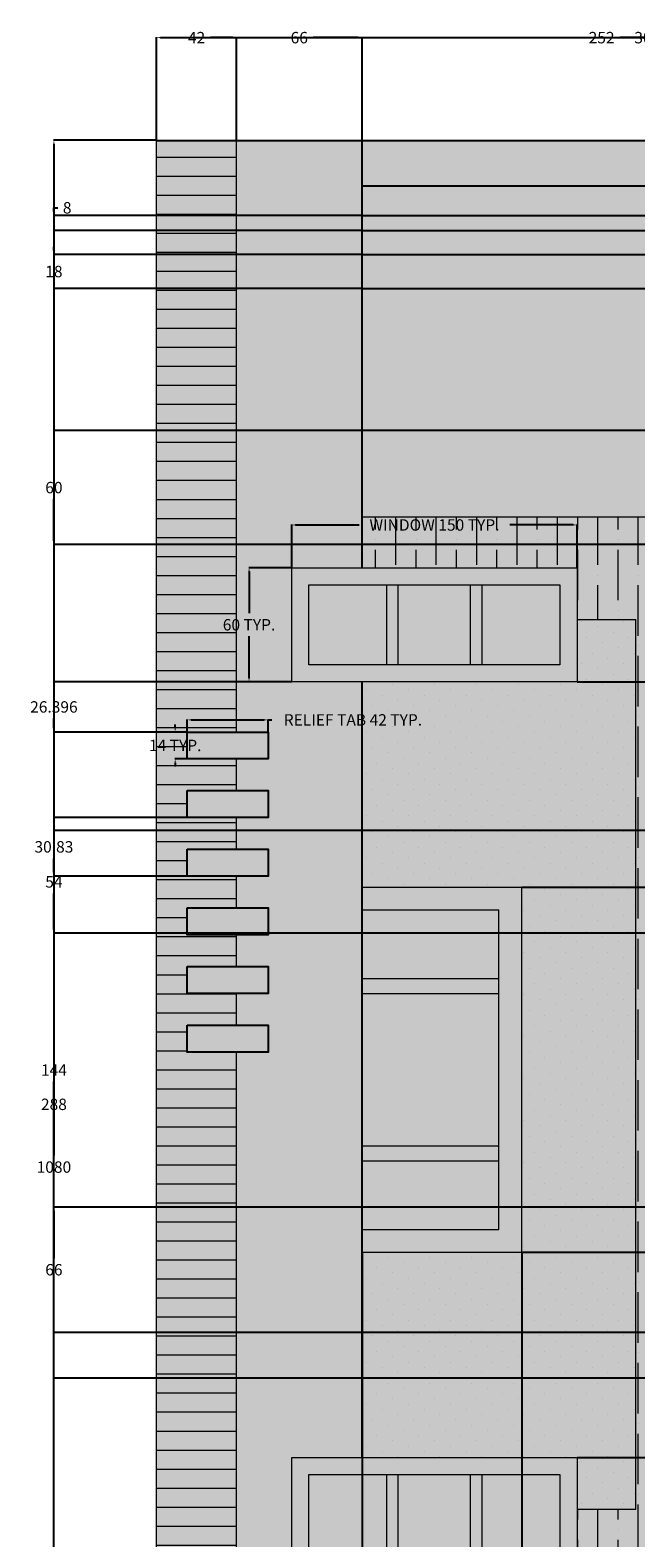
# Model space of a CAD drawing. Units: inches. Extents: x 180 to 1069, y 71 to 1267.
# Tile 6 of 8: x 180 to 498, y 474 to 1267. Entities that reach past the tile are written whole.
import ezdxf

# ---------------------------------------------------------------- set-up
doc = ezdxf.new("R2010")
doc.units = ezdxf.units.IN
doc.header["$MEASUREMENT"] = 0
for name, color, linetype, lineweight in [('A-ANNO-DIMS', 2, 'Continuous', 18), ('A-ELEV-FRAM', 7, 'Continuous', 25), ('A-GLAZ', 7, 'Continuous', 18), ('A-WALL-CLAD', 7, 'Continuous', 18), ('A-WALL-CLAD-JNTS-PATT', 18, 'Continuous', 13), ('A-WALL-CLAD-PATT', 26, 'Continuous', 13), ('A-WALL-SCRN-JNTS-PATT', 8, 'Continuous', 13)]:
    doc.layers.add(name, color=color, linetype=linetype, lineweight=lineweight)
for name, color, linetype, lineweight, true_color in [('A-ELEV-BAND-PATT', 30, 'Continuous', 13, 0xf26722), ('A-ELEV-FRAM-PATT', 53, 'Continuous', 13, 0xefd648), ('A-ELEV-REVL-PATT', 9, 'Continuous', 13, 0xc7c8ca), ('A-ELEV-TRIM-PATT', 7, 'Continuous', 13, 0xffffff), ('A-WALL-PANL-PATT', 252, 'Continuous', 13, 0x939598), ('A-WALL-SCRN-PATT', 251, 'Continuous', 13, 0x636466), ('A-WALL-STUC-PATT', 9, 'Continuous', 13, 0xc7c8ca)]:
    doc.layers.add(name, color=color, linetype=linetype, lineweight=lineweight, true_color=true_color)
doc.styles.get("Standard").update_dxf_attribs({"font": 'arial.ttf'})
doc.dimstyles.get("Standard").update_dxf_attribs({"dimtxt": 6, "dimasz": 2, "dimexe": 0.18, "dimexo": 0.0625, "dimgap": 3, "dimtad": 0, "dimtih": 1, "dimtoh": 1, "dimdec": 0, "dimzin": 0, "dimdsep": 46, "dimlunit": 3, "dimtxsty": 'Standard', "dimcen": 0.09, "dimadec": 0, "dimazin": 0, "dimtfac": 1, "dimtdec": 0, "dimtofl": 0, "dimtmove": 0, "dimatfit": 3, "dimfxl": 1, "dimtolj": 1, "dimtzin": 0, "dimarcsym": 0})

# ---------------------------------------------------------------- blocks, each defined once
blk = doc.blocks.new('WIN-THREE-LIGHT')
for p, q in [((50, 9), (50, 51)), ((56, 9), (56, 51)), ((94, 9), (94, 51)), ((100, 9), (100, 51))]:
    blk.add_line(p, q)
for points in [[(0, 60), (150, 60), (150, 0), (0, 0)], [(9, 51), (141, 51), (141, 9), (9, 9)]]:
    blk.add_lwpolyline(points, close=True)
blk = doc.blocks.new('FACADE-RELIEF-TAB')
blk.add_lwpolyline([(0, 14.15), (42.5, 14.15), (42.5, 0), (0, 0)], close=True)
blk = doc.blocks.new('*D8')
at = {"layer": 'A-ANNO-DIMS', "color": 0, "lineweight": -2, "transparency": 16777216}
for p, q in [((262.22, 897.7), (262.22, 904.19)), ((264.22, 904.01), (302.72, 904.01)), ((304.72, 897.7), (304.72, 904.19)), ((304.72, 904.01), (306.72, 904.01))]:
    blk.add_line(p, q, dxfattribs=at)
at = {"layer": 'A-ANNO-DIMS', "color": 0, "transparency": 16777216}
for points in [[(264.22, 904.34), (264.22, 903.68), (262.22, 904.01)], [(302.72, 904.34), (302.72, 903.68), (304.72, 904.01)]]:
    blk.add_solid(points, dxfattribs=at)
at = {"layer": 'Defpoints', "color": 0, "transparency": 16777216}
for p in [(304.72, 904.01), (262.22, 897.63), (304.72, 897.63)]:
    blk.add_point(p, dxfattribs=at)
at = {"layer": 'A-ANNO-DIMS', "color": 0, "transparency": 16777216, "insert": (349.32, 904.01), "char_height": 6, "attachment_point": 5}
blk.add_mtext('\\A1;RELIEF TAB 42 TYP.', dxfattribs=at)
blk = doc.blocks.new('*D9')
at = {"layer": 'A-ANNO-DIMS', "color": 0, "lineweight": -2, "transparency": 16777216}
for p, q in [((262.16, 897.63), (255.66, 897.63)), ((255.84, 899.63), (255.84, 901.63)), ((262.16, 883.48), (255.66, 883.48)), ((255.84, 881.48), (255.84, 879.48))]:
    blk.add_line(p, q, dxfattribs=at)
at = {"layer": 'A-ANNO-DIMS', "color": 0, "transparency": 16777216}
for points in [[(255.51, 899.63), (256.18, 899.63), (255.84, 897.63)], [(255.51, 881.48), (256.18, 881.48), (255.84, 883.48)]]:
    blk.add_solid(points, dxfattribs=at)
at = {"layer": 'Defpoints', "color": 0, "transparency": 16777216}
for p in [(255.84, 897.63), (262.22, 897.63), (262.22, 883.48)]:
    blk.add_point(p, dxfattribs=at)
at = {"layer": 'A-ANNO-DIMS', "color": 0, "transparency": 16777216, "insert": (255.84, 890.56), "char_height": 6, "attachment_point": 5}
blk.add_mtext('\\A1;14 TYP.', dxfattribs=at)
blk = doc.blocks.new('*D10')
at = {"layer": 'A-ANNO-DIMS', "color": 0, "lineweight": -2, "transparency": 16777216}
for p, q in [((317.19, 984.09), (317.19, 1006.71)), ((319.19, 1006.53), (352.58, 1006.53)), ((465.19, 1006.53), (431.8, 1006.53)), ((467.19, 984.09), (467.19, 1006.71))]:
    blk.add_line(p, q, dxfattribs=at)
at = {"layer": 'A-ANNO-DIMS', "color": 0, "transparency": 16777216}
for points in [[(319.19, 1006.86), (319.19, 1006.2), (317.19, 1006.53)], [(465.19, 1006.86), (465.19, 1006.2), (467.19, 1006.53)]]:
    blk.add_solid(points, dxfattribs=at)
at = {"layer": 'Defpoints', "color": 0, "transparency": 16777216}
for p in [(467.19, 1006.53), (317.19, 984.03), (467.19, 984.03)]:
    blk.add_point(p, dxfattribs=at)
at = {"layer": 'A-ANNO-DIMS', "color": 0, "transparency": 16777216, "insert": (392.19, 1006.53), "char_height": 6, "attachment_point": 5}
blk.add_mtext('\\A1;WINDOW 150 TYP.', dxfattribs=at)
blk = doc.blocks.new('*D11')
at = {"layer": 'A-ANNO-DIMS', "color": 0, "lineweight": -2, "transparency": 16777216}
for p, q in [((317.13, 984.03), (294.51, 984.03)), ((294.69, 982.03), (294.69, 960.09)), ((294.69, 926.03), (294.69, 947.97)), ((317.13, 924.03), (294.51, 924.03))]:
    blk.add_line(p, q, dxfattribs=at)
at = {"layer": 'A-ANNO-DIMS', "color": 0, "transparency": 16777216}
for points in [[(294.36, 982.03), (295.02, 982.03), (294.69, 984.03)], [(294.36, 926.03), (295.02, 926.03), (294.69, 924.03)]]:
    blk.add_solid(points, dxfattribs=at)
at = {"layer": 'Defpoints', "color": 0, "transparency": 16777216}
for p in [(294.69, 984.03), (317.19, 984.03), (317.19, 924.03)]:
    blk.add_point(p, dxfattribs=at)
at = {"layer": 'A-ANNO-DIMS', "color": 0, "transparency": 16777216, "insert": (294.69, 954.03), "char_height": 6, "attachment_point": 5}
blk.add_mtext('\\A1;60 TYP.', dxfattribs=at)
blk = doc.blocks.new('*D16')
at = {"layer": 'A-ANNO-DIMS', "color": 0, "lineweight": -2, "transparency": 16777216}
for p, q in [((246.09, 1208.88), (246.09, 1263.01)), ((248.09, 1262.83), (614.49, 1262.83)), ((1000.09, 1262.83), (633.69, 1262.83)), ((1002.09, 1148.88), (1002.09, 1263.01))]:
    blk.add_line(p, q, dxfattribs=at)
at = {"layer": 'A-ANNO-DIMS', "color": 0, "transparency": 16777216}
for points in [[(248.09, 1263.16), (248.09, 1262.5), (246.09, 1262.83)], [(1000.09, 1263.16), (1000.09, 1262.5), (1002.09, 1262.83)]]:
    blk.add_solid(points, dxfattribs=at)
at = {"layer": 'Defpoints', "color": 0, "transparency": 16777216}
for p in [(1002.09, 1262.83), (246.09, 1208.82), (1002.09, 1148.82)]:
    blk.add_point(p, dxfattribs=at)
at = {"layer": 'A-ANNO-DIMS', "color": 0, "transparency": 16777216, "insert": (624.09, 1262.83), "char_height": 6, "attachment_point": 5}
blk.add_mtext('\\A1;756', dxfattribs=at)
blk = doc.blocks.new('*D17')
at = {"layer": 'A-ANNO-DIMS', "color": 0, "lineweight": -2, "transparency": 16777216}
for p, q in [((246.02, 1208.82), (191.89, 1208.82)), ((192.07, 1206.82), (192.07, 674.88)), ((192.07, 130.82), (192.07, 662.75)), ((246.02, 128.82), (191.89, 128.82))]:
    blk.add_line(p, q, dxfattribs=at)
at = {"layer": 'A-ANNO-DIMS', "color": 0, "transparency": 16777216}
for points in [[(191.74, 1206.82), (192.41, 1206.82), (192.07, 1208.82)], [(191.74, 130.82), (192.41, 130.82), (192.07, 128.82)]]:
    blk.add_solid(points, dxfattribs=at)
at = {"layer": 'Defpoints', "color": 0, "transparency": 16777216}
for p in [(192.07, 1208.82), (246.09, 1208.82), (246.09, 128.82)]:
    blk.add_point(p, dxfattribs=at)
at = {"layer": 'A-ANNO-DIMS', "color": 0, "transparency": 16777216, "insert": (192.07, 668.82), "char_height": 6, "attachment_point": 5}
blk.add_mtext('\\A1;1080', dxfattribs=at)
blk = doc.blocks.new('*D19')
at = {"layer": 'A-ANNO-DIMS', "color": 0, "lineweight": -2, "transparency": 16777216}
for p, q in [((246.09, 1208.88), (246.09, 1263.01)), ((248.09, 1262.83), (259.7, 1262.83)), ((286.09, 1262.83), (274.47, 1262.83)), ((288.09, 1208.88), (288.09, 1263.01))]:
    blk.add_line(p, q, dxfattribs=at)
at = {"layer": 'A-ANNO-DIMS', "color": 0, "transparency": 16777216}
for points in [[(248.09, 1263.16), (248.09, 1262.5), (246.09, 1262.83)], [(286.09, 1263.16), (286.09, 1262.5), (288.09, 1262.83)]]:
    blk.add_solid(points, dxfattribs=at)
at = {"layer": 'Defpoints', "color": 0, "transparency": 16777216}
for p in [(288.09, 1262.83), (246.09, 1208.82), (288.09, 1208.82)]:
    blk.add_point(p, dxfattribs=at)
at = {"layer": 'A-ANNO-DIMS', "color": 0, "transparency": 16777216, "insert": (267.09, 1262.83), "char_height": 6, "attachment_point": 5}
blk.add_mtext('\\A1;42', dxfattribs=at)
blk = doc.blocks.new('*D20')
at = {"layer": 'A-ANNO-DIMS', "color": 0, "lineweight": -2, "transparency": 16777216}
for p, q in [((288.09, 1208.88), (288.09, 1263.01)), ((290.09, 1262.83), (313.78, 1262.83)), ((352.09, 1262.83), (328.4, 1262.83)), ((354.09, 1184.88), (354.09, 1263.01))]:
    blk.add_line(p, q, dxfattribs=at)
at = {"layer": 'A-ANNO-DIMS', "color": 0, "transparency": 16777216}
for points in [[(290.09, 1263.16), (290.09, 1262.5), (288.09, 1262.83)], [(352.09, 1263.16), (352.09, 1262.5), (354.09, 1262.83)]]:
    blk.add_solid(points, dxfattribs=at)
at = {"layer": 'Defpoints', "color": 0, "transparency": 16777216}
for p in [(354.09, 1262.83), (288.09, 1208.82), (354.09, 1184.82)]:
    blk.add_point(p, dxfattribs=at)
at = {"layer": 'A-ANNO-DIMS', "color": 0, "transparency": 16777216, "insert": (321.09, 1262.83), "char_height": 6, "attachment_point": 5}
blk.add_mtext('\\A1;66', dxfattribs=at)
blk = doc.blocks.new('*D21')
at = {"layer": 'A-ANNO-DIMS', "color": 0, "lineweight": -2, "transparency": 16777216}
for p, q in [((354.09, 1184.88), (354.09, 1263.01)), ((356.09, 1262.83), (494.47, 1262.83)), ((652.09, 1262.83), (513.7, 1262.83)), ((654.09, 1184.88), (654.09, 1263.01))]:
    blk.add_line(p, q, dxfattribs=at)
at = {"layer": 'A-ANNO-DIMS', "color": 0, "transparency": 16777216}
for points in [[(356.09, 1263.16), (356.09, 1262.5), (354.09, 1262.83)], [(652.09, 1263.16), (652.09, 1262.5), (654.09, 1262.83)]]:
    blk.add_solid(points, dxfattribs=at)
at = {"layer": 'Defpoints', "color": 0, "transparency": 16777216}
for p in [(654.09, 1262.83), (354.09, 1184.82), (654.09, 1184.82)]:
    blk.add_point(p, dxfattribs=at)
at = {"layer": 'A-ANNO-DIMS', "color": 0, "transparency": 16777216, "insert": (504.09, 1262.83), "char_height": 6, "attachment_point": 5}
blk.add_mtext('\\A1;300', dxfattribs=at)
blk = doc.blocks.new('*D25')
at = {"layer": 'A-ANNO-DIMS', "color": 0, "lineweight": -2, "transparency": 16777216}
for p, q in [((354.02, 1169.34), (191.89, 1169.34)), ((192.07, 1171.34), (192.07, 1173.34)), ((192.07, 1173.34), (194.07, 1173.34)), ((354.02, 1161.34), (191.89, 1161.34)), ((192.07, 1159.34), (192.07, 1157.34))]:
    blk.add_line(p, q, dxfattribs=at)
at = {"layer": 'A-ANNO-DIMS', "color": 0, "transparency": 16777216}
for points in [[(191.74, 1171.34), (192.41, 1171.34), (192.07, 1169.34)], [(191.74, 1159.34), (192.41, 1159.34), (192.07, 1161.34)]]:
    blk.add_solid(points, dxfattribs=at)
at = {"layer": 'Defpoints', "color": 0, "transparency": 16777216}
for p in [(192.07, 1169.34), (354.09, 1169.34), (354.09, 1161.34)]:
    blk.add_point(p, dxfattribs=at)
at = {"layer": 'A-ANNO-DIMS', "color": 0, "transparency": 16777216, "insert": (199.05, 1173.34), "char_height": 6, "attachment_point": 5}
blk.add_mtext('\\A1;8', dxfattribs=at)
blk = doc.blocks.new('*D27')
at = {"layer": 'A-ANNO-DIMS', "color": 0, "lineweight": -2, "transparency": 16777216}
for p, q in [((192.07, 1150.82), (192.07, 1152.82)), ((354.02, 1148.82), (191.89, 1148.82)), ((354.02, 1130.82), (191.89, 1130.82)), ((192.07, 1128.82), (192.07, 1126.82))]:
    blk.add_line(p, q, dxfattribs=at)
at = {"layer": 'A-ANNO-DIMS', "color": 0, "transparency": 16777216}
for points in [[(191.74, 1150.82), (192.41, 1150.82), (192.07, 1148.82)], [(191.74, 1128.82), (192.41, 1128.82), (192.07, 1130.82)]]:
    blk.add_solid(points, dxfattribs=at)
at = {"layer": 'Defpoints', "color": 0, "transparency": 16777216}
for p in [(192.07, 1148.82), (354.09, 1148.82), (354.09, 1130.82)]:
    blk.add_point(p, dxfattribs=at)
at = {"layer": 'A-ANNO-DIMS', "color": 0, "transparency": 16777216, "insert": (192.07, 1139.82), "char_height": 6, "attachment_point": 5}
blk.add_mtext('\\A1;18', dxfattribs=at)
blk = doc.blocks.new('*D48')
at = {"layer": 'A-ANNO-DIMS', "color": 0, "lineweight": -2, "transparency": 16777216}
for p, q in [((262.16, 852.65), (191.89, 852.65)), ((192.07, 850.65), (192.07, 843.3)), ((192.07, 823.82), (192.07, 831.17)), ((262.16, 821.82), (191.89, 821.82))]:
    blk.add_line(p, q, dxfattribs=at)
at = {"layer": 'A-ANNO-DIMS', "color": 0, "transparency": 16777216}
for points in [[(191.74, 850.65), (192.41, 850.65), (192.07, 852.65)], [(191.74, 823.82), (192.41, 823.82), (192.07, 821.82)]]:
    blk.add_solid(points, dxfattribs=at)
at = {"layer": 'Defpoints', "color": 0, "transparency": 16777216}
for p in [(262.22, 852.65), (192.07, 821.82), (262.22, 821.82)]:
    blk.add_point(p, dxfattribs=at)
at = {"layer": 'A-ANNO-DIMS', "color": 0, "transparency": 16777216, "insert": (192.07, 837.23), "char_height": 6, "attachment_point": 5}
blk.add_mtext('\\A1;30.83', dxfattribs=at)
blk = doc.blocks.new('*D49')
at = {"layer": 'A-ANNO-DIMS', "color": 0, "lineweight": -2, "transparency": 16777216}
for p, q in [((317.13, 924.03), (191.89, 924.03)), ((192.07, 922.03), (192.07, 916.9)), ((192.07, 899.63), (192.07, 904.77)), ((262.16, 897.63), (191.89, 897.63))]:
    blk.add_line(p, q, dxfattribs=at)
at = {"layer": 'A-ANNO-DIMS', "color": 0, "transparency": 16777216}
for points in [[(191.74, 922.03), (192.41, 922.03), (192.07, 924.03)], [(191.74, 899.63), (192.41, 899.63), (192.07, 897.63)]]:
    blk.add_solid(points, dxfattribs=at)
at = {"layer": 'Defpoints', "color": 0, "transparency": 16777216}
for p in [(192.07, 924.03), (317.19, 924.03), (262.22, 897.63)]:
    blk.add_point(p, dxfattribs=at)
at = {"layer": 'A-ANNO-DIMS', "color": 0, "transparency": 16777216, "insert": (192.07, 910.83), "char_height": 6, "attachment_point": 5}
blk.add_mtext('\\A1;26.396', dxfattribs=at)
blk = doc.blocks.new('*D51')
at = {"layer": 'A-ANNO-DIMS', "color": 0, "lineweight": -2, "transparency": 16777216}
for p, q in [((354.09, 624.01), (354.09, 74.62)), ((317.19, 456.06), (317.19, 74.62)), ((319.19, 74.8), (324.84, 74.8)), ((352.09, 74.8), (346.44, 74.8))]:
    blk.add_line(p, q, dxfattribs=at)
at = {"layer": 'A-ANNO-DIMS', "color": 0, "transparency": 16777216}
for points in [[(319.19, 75.14), (319.19, 74.47), (317.19, 74.8)], [(352.09, 75.14), (352.09, 74.47), (354.09, 74.8)]]:
    blk.add_solid(points, dxfattribs=at)
at = {"layer": 'Defpoints', "color": 0, "transparency": 16777216}
for p in [(354.09, 624.07), (317.19, 456.12), (354.09, 74.8)]:
    blk.add_point(p, dxfattribs=at)
at = {"layer": 'A-ANNO-DIMS', "color": 0, "transparency": 16777216, "insert": (335.64, 74.8), "char_height": 6, "attachment_point": 5}
blk.add_mtext('\\A1;36.9', dxfattribs=at)
blk = doc.blocks.new('*D52')
at = {"layer": 'A-ANNO-DIMS', "color": 0, "lineweight": -2, "transparency": 16777216}
for p, q in [((354.09, 624.01), (354.09, 74.62)), ((438.09, 624.01), (438.09, 74.62)), ((356.09, 74.8), (388.8, 74.8)), ((436.09, 74.8), (403.38, 74.8))]:
    blk.add_line(p, q, dxfattribs=at)
at = {"layer": 'A-ANNO-DIMS', "color": 0, "transparency": 16777216}
for points in [[(356.09, 75.14), (356.09, 74.47), (354.09, 74.8)], [(436.09, 75.14), (436.09, 74.47), (438.09, 74.8)]]:
    blk.add_solid(points, dxfattribs=at)
at = {"layer": 'Defpoints', "color": 0, "transparency": 16777216}
for p in [(354.09, 624.07), (438.09, 624.07), (438.09, 74.8)]:
    blk.add_point(p, dxfattribs=at)
at = {"layer": 'A-ANNO-DIMS', "color": 0, "transparency": 16777216, "insert": (396.09, 74.8), "char_height": 6, "attachment_point": 5}
blk.add_mtext('\\A1;84', dxfattribs=at)
blk = doc.blocks.new('*D53')
at = {"layer": 'A-ANNO-DIMS', "color": 0, "lineweight": -2, "transparency": 16777216}
for p, q in [((438.15, 624.07), (1056.28, 624.07)), ((1056.1, 622.07), (1056.1, 576.16)), ((1056.1, 518.12), (1056.1, 564.03)), ((467.25, 516.12), (1056.28, 516.12))]:
    blk.add_line(p, q, dxfattribs=at)
at = {"layer": 'A-ANNO-DIMS', "color": 0, "transparency": 16777216}
for points in [[(1055.77, 622.07), (1056.43, 622.07), (1056.1, 624.07)], [(1055.77, 518.12), (1056.43, 518.12), (1056.1, 516.12)]]:
    blk.add_solid(points, dxfattribs=at)
at = {"layer": 'Defpoints', "color": 0, "transparency": 16777216}
for p in [(438.09, 624.07), (1056.1, 624.07), (467.19, 516.12)]:
    blk.add_point(p, dxfattribs=at)
at = {"layer": 'A-ANNO-DIMS', "color": 0, "transparency": 16777216, "insert": (1056.1, 570.1), "char_height": 6, "attachment_point": 5}
blk.add_mtext('\\A1;107.96', dxfattribs=at)
blk = doc.blocks.new('*D54')
at = {"layer": 'A-ANNO-DIMS', "color": 0, "lineweight": -2, "transparency": 16777216}
for p, q in [((438.15, 816.07), (1056.28, 816.07)), ((1056.1, 814.07), (1056.1, 726.14)), ((1056.1, 626.07), (1056.1, 714.01)), ((438.15, 624.07), (1056.28, 624.07))]:
    blk.add_line(p, q, dxfattribs=at)
at = {"layer": 'A-ANNO-DIMS', "color": 0, "transparency": 16777216}
for points in [[(1055.77, 814.07), (1056.43, 814.07), (1056.1, 816.07)], [(1055.77, 626.07), (1056.43, 626.07), (1056.1, 624.07)]]:
    blk.add_solid(points, dxfattribs=at)
at = {"layer": 'Defpoints', "color": 0, "transparency": 16777216}
for p in [(438.09, 816.07), (1056.1, 816.07), (438.09, 624.07)]:
    blk.add_point(p, dxfattribs=at)
at = {"layer": 'A-ANNO-DIMS', "color": 0, "transparency": 16777216, "insert": (1056.1, 720.07), "char_height": 6, "attachment_point": 5}
blk.add_mtext('\\A1;192', dxfattribs=at)
blk = doc.blocks.new('*D55')
at = {"layer": 'A-ANNO-DIMS', "color": 0, "lineweight": -2, "transparency": 16777216}
for p, q in [((467.25, 924.03), (1056.28, 924.03)), ((1056.1, 922.03), (1056.1, 876.12)), ((1056.1, 818.07), (1056.1, 863.99)), ((438.15, 816.07), (1056.28, 816.07))]:
    blk.add_line(p, q, dxfattribs=at)
at = {"layer": 'A-ANNO-DIMS', "color": 0, "transparency": 16777216}
for points in [[(1055.77, 922.03), (1056.43, 922.03), (1056.1, 924.03)], [(1055.77, 818.07), (1056.43, 818.07), (1056.1, 816.07)]]:
    blk.add_solid(points, dxfattribs=at)
at = {"layer": 'Defpoints', "color": 0, "transparency": 16777216}
for p in [(467.19, 924.03), (1056.1, 924.03), (438.09, 816.07)]:
    blk.add_point(p, dxfattribs=at)
at = {"layer": 'A-ANNO-DIMS', "color": 0, "transparency": 16777216, "insert": (1056.1, 870.05), "char_height": 6, "attachment_point": 5}
blk.add_mtext('\\A1;107.96', dxfattribs=at)
blk = doc.blocks.new('*D57')
at = {"layer": 'A-ANNO-DIMS', "color": 0, "lineweight": -2, "transparency": 16777216}
for p, q in [((354.09, 1010.88), (354.09, 1263.01)), ((356.09, 1262.83), (470.44, 1262.83)), ((604.09, 1262.83), (489.74, 1262.83)), ((606.09, 1010.88), (606.09, 1263.01))]:
    blk.add_line(p, q, dxfattribs=at)
at = {"layer": 'A-ANNO-DIMS', "color": 0, "transparency": 16777216}
for points in [[(356.09, 1263.16), (356.09, 1262.5), (354.09, 1262.83)], [(604.09, 1263.16), (604.09, 1262.5), (606.09, 1262.83)]]:
    blk.add_solid(points, dxfattribs=at)
at = {"layer": 'Defpoints', "color": 0, "transparency": 16777216}
for p in [(606.09, 1262.83), (354.09, 1010.82), (606.09, 1010.82)]:
    blk.add_point(p, dxfattribs=at)
at = {"layer": 'A-ANNO-DIMS', "color": 0, "transparency": 16777216, "insert": (480.09, 1262.83), "char_height": 6, "attachment_point": 5}
blk.add_mtext('\\A1;252', dxfattribs=at)
blk = doc.blocks.new('*D62')
at = {"layer": 'A-ANNO-DIMS', "color": 0, "lineweight": -2, "transparency": 16777216}
for p, q in [((882.02, 1056.2), (191.89, 1056.2)), ((192.07, 1054.2), (192.07, 1032.26)), ((192.07, 998.2), (192.07, 1020.14)), ((882.02, 996.2), (191.89, 996.2))]:
    blk.add_line(p, q, dxfattribs=at)
at = {"layer": 'A-ANNO-DIMS', "color": 0, "transparency": 16777216}
for points in [[(191.74, 1054.2), (192.41, 1054.2), (192.07, 1056.2)], [(191.74, 998.2), (192.41, 998.2), (192.07, 996.2)]]:
    blk.add_solid(points, dxfattribs=at)
at = {"layer": 'Defpoints', "color": 0, "transparency": 16777216}
for p in [(192.07, 1056.2), (882.09, 1056.2), (882.09, 996.2)]:
    blk.add_point(p, dxfattribs=at)
at = {"layer": 'A-ANNO-DIMS', "color": 0, "transparency": 16777216, "insert": (192.07, 1026.2), "char_height": 6, "attachment_point": 5}
blk.add_mtext('\\A1;60', dxfattribs=at)
blk = doc.blocks.new('*D64')
at = {"layer": 'A-ANNO-DIMS', "color": 0, "lineweight": -2, "transparency": 16777216}
for p, q in [((612.46, 845.82), (191.89, 845.82)), ((192.07, 843.82), (192.07, 707.88)), ((192.07, 559.82), (192.07, 695.75)), ((612.46, 557.82), (191.89, 557.82))]:
    blk.add_line(p, q, dxfattribs=at)
at = {"layer": 'A-ANNO-DIMS', "color": 0, "transparency": 16777216}
for points in [[(191.74, 843.82), (192.41, 843.82), (192.07, 845.82)], [(191.74, 559.82), (192.41, 559.82), (192.07, 557.82)]]:
    blk.add_solid(points, dxfattribs=at)
at = {"layer": 'Defpoints', "color": 0, "transparency": 16777216}
for p in [(192.07, 845.82), (612.53, 845.82), (612.53, 557.82)]:
    blk.add_point(p, dxfattribs=at)
at = {"layer": 'A-ANNO-DIMS', "color": 0, "transparency": 16777216, "insert": (192.07, 701.82), "char_height": 6, "attachment_point": 5}
blk.add_mtext('\\A1;288', dxfattribs=at)
blk = doc.blocks.new('*D71')
at = {"layer": 'A-ANNO-DIMS', "color": 0, "lineweight": -2, "transparency": 16777216}
for p, q in [((978.02, 647.82), (191.89, 647.82)), ((192.07, 645.82), (192.07, 620.88)), ((192.07, 583.82), (192.07, 608.75)), ((978.02, 581.82), (191.89, 581.82))]:
    blk.add_line(p, q, dxfattribs=at)
at = {"layer": 'A-ANNO-DIMS', "color": 0, "transparency": 16777216}
for points in [[(191.74, 645.82), (192.41, 645.82), (192.07, 647.82)], [(191.74, 583.82), (192.41, 583.82), (192.07, 581.82)]]:
    blk.add_solid(points, dxfattribs=at)
at = {"layer": 'Defpoints', "color": 0, "transparency": 16777216}
for p in [(192.07, 647.82), (978.09, 647.82), (978.09, 581.82)]:
    blk.add_point(p, dxfattribs=at)
at = {"layer": 'A-ANNO-DIMS', "color": 0, "transparency": 16777216, "insert": (192.07, 614.82), "char_height": 6, "attachment_point": 5}
blk.add_mtext('\\A1;66', dxfattribs=at)
blk = doc.blocks.new('*D72')
at = {"layer": 'A-ANNO-DIMS', "color": 0, "lineweight": -2, "transparency": 16777216}
for p, q in [((978.02, 791.82), (191.89, 791.82)), ((192.07, 789.82), (192.07, 725.83)), ((192.07, 649.82), (192.07, 713.8)), ((978.02, 647.82), (191.89, 647.82))]:
    blk.add_line(p, q, dxfattribs=at)
at = {"layer": 'A-ANNO-DIMS', "color": 0, "transparency": 16777216}
for points in [[(191.74, 789.82), (192.41, 789.82), (192.07, 791.82)], [(191.74, 649.82), (192.41, 649.82), (192.07, 647.82)]]:
    blk.add_solid(points, dxfattribs=at)
at = {"layer": 'Defpoints', "color": 0, "transparency": 16777216}
for p in [(192.07, 791.82), (978.09, 791.82), (978.09, 647.82)]:
    blk.add_point(p, dxfattribs=at)
at = {"layer": 'A-ANNO-DIMS', "color": 0, "transparency": 16777216, "insert": (192.07, 719.82), "char_height": 6, "attachment_point": 5}
blk.add_mtext('\\A1;144', dxfattribs=at)
blk = doc.blocks.new('*D73')
at = {"layer": 'A-ANNO-DIMS', "color": 0, "lineweight": -2, "transparency": 16777216}
for p, q in [((978.02, 845.82), (191.89, 845.82)), ((192.07, 843.82), (192.07, 824.87)), ((192.07, 793.82), (192.07, 812.76)), ((978.02, 791.82), (191.89, 791.82))]:
    blk.add_line(p, q, dxfattribs=at)
at = {"layer": 'A-ANNO-DIMS', "color": 0, "transparency": 16777216}
for points in [[(191.74, 843.82), (192.41, 843.82), (192.07, 845.82)], [(191.74, 793.82), (192.41, 793.82), (192.07, 791.82)]]:
    blk.add_solid(points, dxfattribs=at)
at = {"layer": 'Defpoints', "color": 0, "transparency": 16777216}
for p in [(192.07, 845.82), (978.09, 845.82), (978.09, 791.82)]:
    blk.add_point(p, dxfattribs=at)
at = {"layer": 'A-ANNO-DIMS', "color": 0, "transparency": 16777216, "insert": (192.07, 818.82), "char_height": 6, "attachment_point": 5}
blk.add_mtext('\\A1;54', dxfattribs=at)

msp = doc.modelspace()

# ---------------------------------------------------------------- hatches: boundary and pattern name
at = {"layer": 'A-ELEV-BAND-PATT'}
h = msp.add_hatch(color=256, dxfattribs=at)
h.dxf.hatch_style = 1
h.paths.add_polyline_path([(1002.0875, 1148.8159), (726.0875, 1148.8159), (726.0875, 1130.8159), (954.0875, 1130.8159), (954.0875, 947.2513), (978.0875, 947.2513), (978.0875, 1130.8159), (1002.0875, 1130.8159)])
h.paths.add_polyline_path([(654.0875, 1148.8159), (354.0875, 1148.8159), (354.0875, 1130.8159), (654.0875, 1130.8159)])
h.paths.add_polyline_path([(606.0875, 434.8159), (246.0875, 434.8159), (246.0875, 416.8159), (606.0875, 416.8159)])
h.paths.add_polyline_path([(978.0875, 845.8159), (726.0875, 845.8159), (726.0875, 791.8159), (978.0875, 791.8159)])
at = {"layer": 'A-ELEV-FRAM-PATT'}
h = msp.add_hatch(color=256, dxfattribs=at)
h.dxf.hatch_style = 1
h.paths.add_polyline_path([(354.0875, 1184.8159), (654.0875, 1184.8159), (654.0875, 974.8159), (726.0875, 974.8159), (726.0875, 1208.8159), (288.0875, 1208.8159), (288.0875, 897.6348), (304.7188, 897.6348), (304.7188, 883.4805), (288.0875, 883.4805), (288.0875, 866.8025), (304.7188, 866.8025), (304.7188, 852.6482), (288.0875, 852.6482), (288.0875, 835.9702), (304.7188, 835.9702), (304.7188, 821.8159), (288.0875, 821.8159), (288.0875, 805.1379), (304.7188, 805.1379), (304.7188, 790.9836), (288.0875, 790.9836), (288.0875, 774.3056), (304.7188, 774.3056), (304.7188, 760.1513), (288.0875, 760.1513), (288.0875, 743.4733), (304.7188, 743.4733), (304.7188, 729.319), (288.0875, 729.319), (288.0875, 434.8159), (354.0875, 434.8159), (354.0875, 456.1177), (317.1892, 456.1177), (317.1892, 516.1177), (354.0875, 516.1177), (354.0875, 924.0304), (317.1892, 924.0304), (317.1892, 984.0304), (354.0875, 984.0304)])
h.paths.add_polyline_path([(1002.0875, 869.8159), (702.0875, 869.8159), (702.0875, 791.8159), (726.0875, 791.8159), (726.0875, 845.8159), (978.0875, 845.8159), (978.0875, 581.8159), (726.0875, 581.8159), (726.0875, 647.8159), (702.0875, 647.8159), (702.0875, 557.8159), (1002.0875, 557.8159)])
h.paths.add_polyline_path([(906.0875, 1080.2003), (882.0875, 1080.2003), (882.0875, 1056.2003), (906.0875, 1056.2003)])
h.paths.add_polyline_path([(906.0875, 996.2003), (882.0875, 996.2003), (882.0875, 972.2003), (906.0875, 972.2003)])
h.paths.add_polyline_path([(636.5273, 869.8159), (612.5273, 869.8159), (612.5273, 845.8159), (636.5273, 845.8159)], flags=17)
h.paths.add_polyline_path([(682.6602, 869.8159), (658.6602, 869.8159), (658.6602, 845.8159), (682.6602, 845.8159)], flags=17)
h.paths.add_polyline_path([(636.5273, 581.8159), (612.5273, 581.8159), (612.5273, 557.8159), (636.5273, 557.8159)], flags=17)
h.paths.add_polyline_path([(682.6602, 581.8159), (658.6602, 581.8159), (658.6602, 557.8159), (682.6602, 557.8159)], flags=17)
h.paths.add_polyline_path([(942.0875, 358.0477), (918.0875, 358.0477), (918.0875, 128.8159), (942.0875, 128.8159)])
h.paths.add_polyline_path([(630.0875, 358.0477), (606.0875, 358.0477), (606.0875, 128.8159), (630.0875, 128.8159)])
at = {"layer": 'A-ELEV-REVL-PATT'}
h = msp.add_hatch(color=256, dxfattribs=at)
h.dxf.hatch_style = 1
h.paths.add_polyline_path([(654.0875, 1161.3367), (654.0875, 1169.3367), (354.0875, 1169.3367), (354.0875, 1161.3367)])
h = msp.add_hatch(color=256, dxfattribs=at)
h.dxf.hatch_style = 1
h.paths.add_polyline_path([(426.0875, 680.0741), (354.0875, 680.0741), (354.0875, 672.0741), (426.0875, 672.0741)])
h.paths.add_polyline_path([(426.0875, 768.0741), (354.0875, 768.0741), (354.0875, 760.0741), (426.0875, 760.0741)])
h.paths.add_polyline_path([(417.1892, 507.1177), (411.1892, 507.1177), (411.1892, 465.1177), (417.1892, 465.1177)])
h.paths.add_polyline_path([(373.1892, 507.1177), (367.1892, 507.1177), (367.1892, 465.1177), (373.1892, 465.1177)])
h.paths.add_polyline_path([(373.1892, 975.0304), (367.1892, 975.0304), (367.1892, 933.0304), (373.1892, 933.0304)])
h.paths.add_polyline_path([(417.1892, 975.0304), (411.1892, 975.0304), (411.1892, 933.0304), (417.1892, 933.0304)])
at = {"layer": 'A-ELEV-TRIM-PATT'}
h = msp.add_hatch(color=256, dxfattribs=at)
h.dxf.hatch_style = 1
h.paths.add_polyline_path([(654.0875, 1130.8159), (354.0875, 1130.8159), (354.0875, 1010.8159), (606.0875, 1010.8159), (606.0875, 974.8159), (654.0875, 974.8159)])
h.paths.add_polyline_path([(654.0875, 1161.3367), (354.0875, 1161.3367), (354.0875, 1148.8159), (654.0875, 1148.8159)])
h.paths.add_polyline_path([(654.0875, 1184.8159), (354.0875, 1184.8159), (354.0875, 1169.3367), (654.0875, 1169.3367)])
h.paths.add_polyline_path([(954.0875, 1130.8159), (726.0875, 1130.8159), (726.0875, 974.8159), (834.0875, 974.8159), (834.0875, 947.2513), (954.0875, 947.2513)])
h.paths.add_polyline_path([(882.0875, 1056.2003), (882.0875, 1080.2003), (906.0875, 1080.2003), (906.0875, 1056.2003)], flags=16)
h.paths.add_polyline_path([(882.0875, 996.2003), (906.0875, 996.2003), (906.0875, 972.2003), (882.0875, 972.2003)], flags=16)
h = msp.add_hatch(color=256, dxfattribs=at)
h.dxf.hatch_style = 1
h.paths.add_polyline_path([(467.1892, 516.1177), (317.1892, 516.1177), (317.1892, 456.1177), (467.1892, 456.1177)])
h.paths.add_polyline_path([(458.1892, 507.1177), (458.1892, 465.1177), (326.1892, 465.1177), (326.1892, 507.1177)], flags=16)
h.paths.add_polyline_path([(354.0875, 816.0741), (354.0875, 804.0741), (426.0875, 804.0741), (426.0875, 636.0741), (354.0875, 636.0741), (354.0875, 624.0741), (438.0875, 624.0741), (438.0875, 816.0741)])
h.paths.add_polyline_path([(317.1892, 924.0304), (467.1892, 924.0304), (467.1892, 984.0304), (317.1892, 984.0304)])
h.paths.add_polyline_path([(326.1892, 933.0304), (326.1892, 975.0304), (458.1892, 975.0304), (458.1892, 933.0304)], flags=16)
h.paths.add_polyline_path([(304.7188, 897.6348), (262.2193, 897.6348), (262.2193, 883.4805), (304.7188, 883.4805)])
h.paths.add_polyline_path([(304.7188, 866.8025), (262.2193, 866.8025), (262.2193, 852.6482), (304.7188, 852.6482)])
h.paths.add_polyline_path([(304.7188, 835.9702), (262.2193, 835.9702), (262.2193, 821.8159), (304.7188, 821.8159)])
h.paths.add_polyline_path([(304.7188, 805.1379), (262.2193, 805.1379), (262.2193, 790.9836), (304.7188, 790.9836)])
h.paths.add_polyline_path([(304.7188, 774.3056), (262.2193, 774.3056), (262.2193, 760.1513), (304.7188, 760.1513)])
h.paths.add_polyline_path([(304.7188, 743.4733), (262.2193, 743.4733), (262.2193, 729.319), (304.7188, 729.319)])
h.paths.add_polyline_path([(600.0875, 370.0477), (600.0875, 358.0477), (636.0875, 358.0477), (636.0875, 370.0477)])
h.paths.add_polyline_path([(912.0875, 370.0477), (912.0875, 358.0477), (948.0875, 358.0477), (948.0875, 370.0477)])
at = {"layer": 'A-WALL-CLAD-JNTS-PATT'}
h = msp.add_hatch(dxfattribs=at)
h.set_pattern_fill('ANSI31', color=256, scale=80, angle=135)
h.paths.add_polyline_path([(288.0875, 416.8159), (246.0875, 416.8159), (246.0875, 128.8159), (288.0875, 128.8159)])
h.paths.add_polyline_path([(606.0875, 358.0477), (600.0875, 358.0477), (600.0875, 370.0477), (606.0875, 370.0477), (606.0875, 416.8159), (564.0875, 416.8159), (564.0875, 128.8159), (606.0875, 128.8159)])
h.paths.add_polyline_path([(288.0875, 729.319), (262.2193, 729.319), (262.2193, 743.4733), (288.0875, 743.4733), (288.0875, 760.1513), (262.2193, 760.1513), (262.2193, 774.3056), (288.0875, 774.3056), (288.0875, 790.9836), (262.2193, 790.9836), (262.2193, 805.1379), (288.0875, 805.1379), (288.0875, 821.8159), (262.2193, 821.8159), (262.2193, 835.9702), (288.0875, 835.9702), (288.0875, 852.6482), (262.2193, 852.6482), (262.2193, 866.8025), (288.0875, 866.8025), (288.0875, 883.4805), (262.2193, 883.4805), (262.2193, 897.6348), (288.0875, 897.6348), (288.0875, 1208.8159), (246.0875, 1208.8159), (246.0875, 434.8159), (288.0875, 434.8159)])
at = {"layer": 'A-WALL-CLAD-PATT'}
h = msp.add_hatch(color=256, dxfattribs=at)
h.dxf.hatch_style = 1
h.paths.add_polyline_path([(288.0875, 1208.8159), (246.0875, 1208.8159), (246.0875, 434.8159), (288.0875, 434.8159), (288.0875, 729.319), (262.2193, 729.319), (262.2193, 743.4733), (288.0875, 743.4733), (288.0875, 760.1513), (262.2193, 760.1513), (262.2193, 774.3056), (288.0875, 774.3056), (288.0875, 790.9836), (262.2193, 790.9836), (262.2193, 805.1379), (288.0875, 805.1379), (288.0875, 821.8159), (262.2193, 821.8159), (262.2193, 835.9702), (288.0875, 835.9702), (288.0875, 852.6482), (262.2193, 852.6482), (262.2193, 866.8025), (288.0875, 866.8025), (288.0875, 883.4805), (262.2193, 883.4805), (262.2193, 897.6348), (288.0875, 897.6348)])
h.paths.add_polyline_path([(288.0875, 416.8159), (246.0875, 416.8159), (246.0875, 128.8159), (288.0875, 128.8159)])
at = {"layer": 'A-WALL-PANL-PATT'}
h = msp.add_hatch(color=256, dxfattribs=at)
h.dxf.hatch_style = 1
h.paths.add_polyline_path([(498.0875, 956.8159), (467.1892, 956.8159), (467.1892, 924.0304), (354.0875, 924.0304), (354.0875, 816.0741), (438.0875, 816.0741), (438.0875, 624.0741), (354.0875, 624.0741), (354.0875, 516.1177), (467.1892, 516.1177), (467.1892, 488.8159), (498.0875, 488.8159)])
h.paths.add_polyline_path([(798.0875, 938.8159), (606.0875, 938.8159), (606.0875, 791.8159), (702.0875, 791.8159), (702.0875, 869.8159), (798.0875, 869.8159)])
h.paths.add_polyline_path([(682.6602, 869.8159), (682.6602, 845.8159), (658.6602, 845.8159), (658.6602, 869.8159)], flags=16)
h.paths.add_polyline_path([(636.5273, 869.8159), (636.5273, 845.8159), (612.5273, 845.8159), (612.5273, 869.8159)], flags=16)
h.paths.add_polyline_path([(702.0875, 647.8159), (606.0875, 647.8159), (606.0875, 509.8159), (798.0875, 509.8159), (798.0875, 557.8159), (702.0875, 557.8159)])
h.paths.add_polyline_path([(658.6602, 581.8159), (682.6602, 581.8159), (682.6602, 557.8159), (658.6602, 557.8159)], flags=16)
h.paths.add_polyline_path([(636.5273, 581.8159), (636.5273, 557.8159), (612.5273, 557.8159), (612.5273, 581.8159)], flags=16)
at = {"layer": 'A-WALL-SCRN-JNTS-PATT'}
h = msp.add_hatch(dxfattribs=at)
h.set_pattern_fill('ANSI36', color=256, scale=85, angle=45)
h.paths.add_polyline_path([(606.0875, 938.8159), (798.0875, 938.8159), (798.0875, 869.8159), (834.0875, 869.8159), (834.0875, 974.8159), (606.0875, 974.8159), (606.0875, 1010.8159), (354.0875, 1010.8159), (354.0875, 984.0304), (467.1892, 984.0304), (467.1892, 956.8159), (498.0875, 956.8159), (498.0875, 488.8159), (467.1892, 488.8159), (467.1892, 456.1177), (354.0875, 456.1177), (354.0875, 434.8159), (606.0875, 434.8159), (606.0875, 473.8159), (834.0875, 473.8159), (834.0875, 557.8159), (798.0875, 557.8159), (798.0875, 509.8159), (606.0875, 509.8159)])
at = {"layer": 'A-WALL-SCRN-PATT'}
h = msp.add_hatch(color=256, dxfattribs=at)
h.dxf.hatch_style = 1
h.paths.add_polyline_path([(606.0875, 938.8159), (798.0875, 938.8159), (798.0875, 869.8159), (834.0875, 869.8159), (834.0875, 974.8159), (606.0875, 974.8159), (606.0875, 1010.8159), (354.0875, 1010.8159), (354.0875, 984.0304), (467.1892, 984.0304), (467.1892, 956.8159), (498.0875, 956.8159), (498.0875, 488.8159), (467.1892, 488.8159), (467.1892, 456.1177), (354.0875, 456.1177), (354.0875, 434.8159), (606.0875, 434.8159), (606.0875, 473.8159), (834.0875, 473.8159), (834.0875, 557.8159), (798.0875, 557.8159), (798.0875, 509.8159), (606.0875, 509.8159)])
h.paths.add_polyline_path([(367.1892, 507.1177), (326.1892, 507.1177), (326.1892, 465.1177), (367.1892, 465.1177)])
h.paths.add_polyline_path([(411.1892, 507.1177), (373.1892, 507.1177), (373.1892, 465.1177), (411.1892, 465.1177)], flags=17)
h.paths.add_polyline_path([(458.1892, 507.1177), (417.1892, 507.1177), (417.1892, 465.1177), (458.1892, 465.1177)], flags=17)
h.paths.add_polyline_path([(426.0875, 672.0741), (354.0875, 672.0741), (354.0875, 636.0741), (426.0875, 636.0741)], flags=17)
h.paths.add_polyline_path([(426.0875, 760.0741), (354.0875, 760.0741), (354.0875, 680.0741), (426.0875, 680.0741)], flags=17)
h.paths.add_polyline_path([(426.0875, 804.0741), (354.0875, 804.0741), (354.0875, 768.0741), (426.0875, 768.0741)], flags=17)
h.paths.add_polyline_path([(367.1892, 975.0304), (326.1892, 975.0304), (326.1892, 933.0304), (367.1892, 933.0304)])
h.paths.add_polyline_path([(411.1892, 975.0304), (373.1892, 975.0304), (373.1892, 933.0304), (411.1892, 933.0304)], flags=17)
h.paths.add_polyline_path([(458.1892, 975.0304), (417.1892, 975.0304), (417.1892, 933.0304), (458.1892, 933.0304)], flags=17)
at = {"layer": 'A-WALL-STUC-PATT'}
h = msp.add_hatch(dxfattribs=at)
h.set_pattern_fill('DOTS', color=256, scale=30, angle=135)
h.paths.add_polyline_path([(654.0875, 1184.8159), (354.0875, 1184.8159), (354.0875, 1169.3367), (654.0875, 1169.3367)])
h.paths.add_polyline_path([(654.0875, 1161.3367), (354.0875, 1161.3367), (354.0875, 1148.8159), (654.0875, 1148.8159)])
h = msp.add_hatch(dxfattribs=at)
h.set_pattern_fill('DOTS', color=256, scale=30, angle=135)
h.paths.add_polyline_path([(654.0875, 1130.8159), (354.0875, 1130.8159), (354.0875, 1010.8159), (606.0875, 1010.8159), (606.0875, 974.8159), (654.0875, 974.8159)])
h.paths.add_polyline_path([(954.0875, 1130.8159), (726.0875, 1130.8159), (726.0875, 974.8159), (834.0875, 974.8159), (834.0875, 947.2513), (954.0875, 947.2513)])
h.paths.add_polyline_path([(882.0875, 1080.2003), (906.0875, 1080.2003), (906.0875, 1056.2003), (882.0875, 1056.2003)], flags=16)
h.paths.add_polyline_path([(882.0875, 996.2003), (906.0875, 996.2003), (906.0875, 972.2003), (882.0875, 972.2003)], flags=16)
h = msp.add_hatch(dxfattribs=at)
h.set_pattern_fill('DOTS', color=256, scale=125, angle=45)
h.paths.add_polyline_path([(498.0875, 956.8159), (467.1892, 956.8159), (467.1892, 924.0304), (354.0875, 924.0304), (354.0875, 816.0741), (438.0875, 816.0741), (438.0875, 624.0741), (354.0875, 624.0741), (354.0875, 516.1177), (467.1892, 516.1177), (467.1892, 488.8159), (498.0875, 488.8159)])

# ---------------------------------------------------------------- linework, layer by layer
at = {"layer": 'A-ELEV-FRAM'}
for p, q in [((246.0875, 1208.8159), (726.0875, 1208.8159)), ((354.0875, 1184.8159), (654.0875, 1184.8159)), ((354.0875, 984.0304), (354.0875, 1184.8159)), ((354.0875, 1169.3367), (654.0875, 1169.3367)), ((354.0875, 1161.3367), (654.0875, 1161.3367)), ((354.0875, 1148.8159), (654.0875, 1148.8159)), ((354.0875, 1130.8159), (654.0875, 1130.8159)), ((354.0875, 516.1177), (354.0875, 924.0304))]:
    msp.add_line(p, q, dxfattribs=at)
at = {"layer": 'A-GLAZ'}
for p, q in [((354.0875, 816.0741), (438.0875, 816.0741)), ((438.0875, 624.0741), (438.0875, 816.0741)), ((354.0875, 804.0741), (426.0875, 804.0741)), ((426.0875, 636.0741), (426.0875, 804.0741)), ((354.0875, 768.0741), (426.0875, 768.0741)), ((354.0875, 760.0741), (426.0875, 760.0741)), ((354.0875, 680.0741), (426.0875, 680.0741)), ((354.0875, 672.0741), (426.0875, 672.0741)), ((354.0875, 636.0741), (426.0875, 636.0741)), ((354.0875, 624.0741), (438.0875, 624.0741))]:
    msp.add_line(p, q, dxfattribs=at)
at = {"layer": 'A-WALL-CLAD'}
for p, q in [((246.0875, 128.8159), (246.0875, 1208.8159)), ((288.0875, 897.6348), (288.0875, 1208.8159)), ((354.0875, 1010.8159), (606.0875, 1010.8159)), ((467.1892, 956.8159), (498.0875, 956.8159)), ((498.0875, 488.8159), (498.0875, 956.8159)), ((288.0875, 866.8025), (288.0875, 883.4805)), ((288.0875, 835.9702), (288.0875, 852.6482)), ((288.0875, 805.1379), (288.0875, 821.8159)), ((288.0875, 774.3056), (288.0875, 790.9836)), ((288.0875, 743.4733), (288.0875, 760.1513)), ((288.0875, 434.8159), (288.0875, 729.319)), ((467.1892, 488.8159), (498.0875, 488.8159))]:
    msp.add_line(p, q, dxfattribs=at)

# ---------------------------------------------------------------- block references
at = {"layer": 'A-ELEV-FRAM'}
for p in [(262.2193, 883.4805), (262.2193, 852.6482), (262.2193, 821.8159), (262.2193, 790.9836), (262.2193, 760.1513), (262.2193, 729.319)]:
    msp.add_blockref('FACADE-RELIEF-TAB', p, dxfattribs=at)
at = {"layer": 'A-GLAZ'}
for p in [(317.1892, 924.0304), (317.1892, 456.1177)]:
    msp.add_blockref('WIN-THREE-LIGHT', p, dxfattribs=at)

# ---------------------------------------------------------------- dimensions: what is measured, and where the dimension line sits
at = {"layer": 'A-ANNO-DIMS'}
for base, p1, p2, override, picture, middle in [((1002.0875, 1262.8294), (246.0875, 1208.8159), (1002.0875, 1148.8159), {"dimdec": 0, "dimlfac": 1, "dimrnd": 0, "dimzin": 0, "dimdsep": 46, "dimlunit": 2}, '*D16', (624.0875, 1262.8294)), ((288.0875, 1262.8294), (246.0875, 1208.8159), (288.0875, 1208.8159), {"dimdec": 0, "dimlfac": 1, "dimrnd": 0, "dimzin": 0, "dimdsep": 46, "dimlunit": 2}, '*D19', (267.0875, 1262.8294)), ((354.0875, 1262.8294), (288.0875, 1208.8159), (354.0875, 1184.8159), {"dimdec": 0, "dimlfac": 1, "dimrnd": 0, "dimzin": 0, "dimdsep": 46, "dimlunit": 2}, '*D20', (321.0875, 1262.8294)), ((654.0875, 1262.8294), (354.0875, 1184.8159), (654.0875, 1184.8159), {"dimdec": 0, "dimlfac": 1, "dimrnd": 0, "dimzin": 0, "dimdsep": 46, "dimlunit": 2}, '*D21', (504.0875, 1262.8294)), ((606.0875, 1262.8294), (354.0875, 1010.8159), (606.0875, 1010.8159), {"dimdec": 0, "dimlfac": 1, "dimrnd": 0, "dimzin": 0, "dimdsep": 46, "dimlunit": 2}, '*D57', (480.0875, 1262.8294)), ((354.0875, 74.8024), (317.1892, 456.1177), (354.0875, 624.0741), {"dimdec": 1, "dimlfac": 1, "dimrnd": 0, "dimzin": 0, "dimdsep": 46, "dimlunit": 2}, '*D51', (335.6383, 74.8024)), ((438.0875, 74.8024), (354.0875, 624.0741), (438.0875, 624.0741), {"dimdec": 0, "dimlfac": 1, "dimrnd": 0, "dimzin": 0, "dimdsep": 46, "dimlunit": 2}, '*D52', (396.0875, 74.8024))]:
    dim = msp.add_linear_dim(base=base, p1=p1, p2=p2, dimstyle='Standard', override=override, dxfattribs=at)
    dim.commit()
    dim.dimension.update_dxf_attribs({"geometry": picture, "text_midpoint": middle})
for base, p1, p2, override, picture, middle in [((192.074, 1208.8159), (246.0875, 128.8159), (246.0875, 1208.8159), {"dimdec": 0, "dimlfac": 1, "dimrnd": 0, "dimzin": 0, "dimdsep": 46, "dimlunit": 2}, '*D17', (192.074, 668.8159)), ((192.074, 1169.3367), (354.0875, 1161.3367), (354.0875, 1169.3367), {"dimdec": 0, "dimlfac": 1, "dimrnd": 0, "dimzin": 0, "dimdsep": 46, "dimlunit": 2}, '*D25', (199.0508, 1173.3367)), ((192.074, 1148.8159), (354.0875, 1130.8159), (354.0875, 1148.8159), {"dimdec": 0, "dimlfac": 1, "dimrnd": 0, "dimzin": 0, "dimdsep": 46, "dimlunit": 2}, '*D27', (192.074, 1139.8159)), ((192.074, 1056.2003), (882.0875, 996.2003), (882.0875, 1056.2003), {"dimdec": 0, "dimlfac": 1, "dimrnd": 0, "dimzin": 0, "dimdsep": 46, "dimlunit": 2}, '*D62', (192.074, 1026.2003)), ((192.074, 924.0304), (262.2193, 897.6348), (317.1892, 924.0304), {"dimdec": 3, "dimlfac": 1, "dimrnd": 0, "dimzin": 0, "dimdsep": 46, "dimlunit": 2}, '*D49', (192.074, 910.8326)), ((1056.101, 924.0304), (438.0875, 816.0741), (467.1892, 924.0304), {"dimdec": 2, "dimlfac": 1, "dimrnd": 0, "dimzin": 0, "dimdsep": 46, "dimlunit": 2}, '*D55', (1056.101, 870.0523)), ((192.074, 821.8159), (262.2193, 852.6482), (262.2193, 821.8159), {"dimdec": 2, "dimlfac": 1, "dimrnd": 0, "dimzin": 0, "dimdsep": 46, "dimlunit": 2}, '*D48', (192.074, 837.232)), ((192.074, 845.8159), (612.5273, 557.8159), (612.5273, 845.8159), {"dimdec": 0, "dimlfac": 1, "dimrnd": 0, "dimzin": 0, "dimdsep": 46, "dimlunit": 2}, '*D64', (192.074, 701.8159)), ((192.074, 845.8159), (978.0875, 791.8159), (978.0875, 845.8159), {"dimdec": 0, "dimlfac": 1, "dimrnd": 0, "dimzin": 0, "dimdsep": 46, "dimlunit": 2}, '*D73', (192.074, 818.8159)), ((1056.101, 816.0741), (438.0875, 624.0741), (438.0875, 816.0741), {"dimdec": 0, "dimlfac": 1, "dimrnd": 0, "dimzin": 0, "dimdsep": 46, "dimlunit": 2}, '*D54', (1056.101, 720.0741)), ((192.074, 791.8159), (978.0875, 647.8159), (978.0875, 791.8159), {"dimdec": 0, "dimlfac": 1, "dimrnd": 0, "dimzin": 0, "dimdsep": 46, "dimlunit": 2}, '*D72', (192.074, 719.8159)), ((192.074, 647.8159), (978.0875, 581.8159), (978.0875, 647.8159), {"dimdec": 0, "dimlfac": 1, "dimrnd": 0, "dimzin": 0, "dimdsep": 46, "dimlunit": 2}, '*D71', (192.074, 614.8159)), ((1056.101, 624.0741), (467.1892, 516.1177), (438.0875, 624.0741), {"dimdec": 2, "dimlfac": 1, "dimrnd": 0, "dimzin": 0, "dimdsep": 46, "dimlunit": 2}, '*D53', (1056.101, 570.0959))]:
    dim = msp.add_linear_dim(base=base, p1=p1, p2=p2, angle=90, dimstyle='Standard', override=override, dxfattribs=at)
    dim.commit()
    dim.dimension.update_dxf_attribs({"geometry": picture, "text_midpoint": middle})
for base, p1, p2, text, picture, middle in [((467.1892, 1006.5304), (317.1892, 984.0304), (467.1892, 984.0304), 'WINDOW <> TYP.', '*D10', (392.1892, 1006.5304)), ((304.7188, 904.0097), (262.2193, 897.6348), (304.7188, 897.6348), 'RELIEF TAB <> TYP.', '*D8', (349.3184, 904.0097))]:
    dim = msp.add_linear_dim(base=base, p1=p1, p2=p2, text=text, dimstyle='Standard', override={"dimdec": 0, "dimlfac": 1, "dimrnd": 0, "dimzin": 0, "dimdsep": 46, "dimlunit": 2}, dxfattribs=at)
    dim.commit()
    dim.dimension.update_dxf_attribs({"geometry": picture, "text_midpoint": middle})
for base, p1, p2, picture, middle in [((294.6892, 984.0304), (317.1892, 924.0304), (317.1892, 984.0304), '*D11', (294.6892, 954.0304)), ((255.8444, 897.6348), (262.2193, 883.4805), (262.2193, 897.6348), '*D9', (255.8444, 890.5576))]:
    dim = msp.add_linear_dim(base=base, p1=p1, p2=p2, angle=90, text='<> TYP.', dimstyle='Standard', override={"dimdec": 0, "dimlfac": 1, "dimrnd": 0, "dimzin": 0, "dimdsep": 46, "dimlunit": 2}, dxfattribs=at)
    dim.commit()
    dim.dimension.update_dxf_attribs({"geometry": picture, "text_midpoint": middle})

doc.saveas('drawing.dxf')
